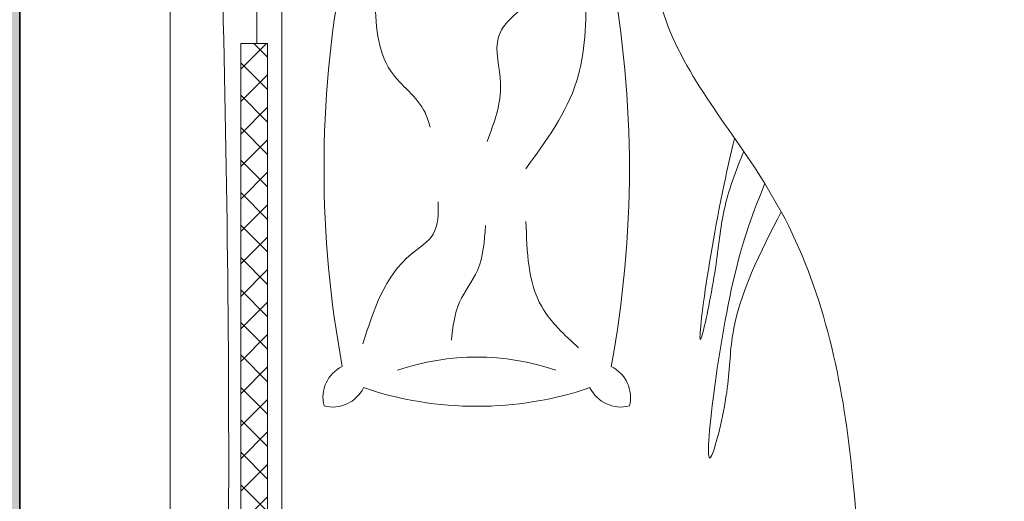
# Model space of a CAD drawing. Units: inches. Extents: x 2083 to 3317, y 1141 to 2115.
# Tile 96 of 256: x 2236 to 2290, y 1932 to 1958. Entities that reach past the tile are written whole.
import ezdxf

# ---------------------------------------------------------------- set-up
doc = ezdxf.new("R2010")
doc.units = ezdxf.units.IN
for name, color, linetype, lineweight in [('A-FURN', 8, 'Continuous', 18), ('A-WALL', 7, 'Continuous', 35), ('www.cadblocksfree.com', 7, 'Continuous', 9)]:
    doc.layers.add(name, color=color, linetype=linetype, lineweight=lineweight)
doc.layers.add('A-WALL-PATT', color=251, linetype='Continuous', lineweight=13, true_color=0x636466)

# ---------------------------------------------------------------- blocks, each defined once
blk = doc.blocks.new('bed')
at = {"layer": 'www.cadblocksfree.com', "ltscale": 0.2}
h = blk.add_hatch(dxfattribs=at)
h.set_pattern_fill('ANSI37,_O', color=256, scale=0.393701)
h.set_pattern_definition([(45, (2420.7222, -262.9689), (-0.8838835, 0.8838835), []), (135, (2420.7222, -262.9689), (-0.8838835, -0.8838835), [])])
h.paths.add_polyline_path([(3417.573, 1472.402), (3372.192, 1472.402), (3372.192, 1470.941), (3417.573, 1470.941)])
for p, q in [((3372.192, 1472.402), (3417.573, 1472.402)), ((3417.573, 1470.941), (3417.573, 1472.402)), ((3372.192, 1470.941), (3417.573, 1470.941)), ((3409.943, 1443.853), (3408.408, 1442.961))]:
    blk.add_line(p, q, dxfattribs=at)
for points in [[(3426.763, 1476.249), (3363.002, 1476.249)], [(3417.573, 1471.524), (3428.347, 1471.524), (3428.347, 1473.886)], [(3426.379, 1449.413), (3426.379, 1470.154), (3363.387, 1470.154), (3363.387, 1447.076)]]:
    blk.add_lwpolyline(points, dxfattribs=at)
for centre, radius, start, end in [((3394.883, 2431.358), 958.303, 268.093559, 271.906441), ((3399.641, 1467.396), 1.87, 165.5166, 244.2099), ((3398.298, 1466.054), 1.87, 25.7901, 104.4834), ((3410.752, 1409.187), 58.677, 79.42346, 100.57654), ((3417.027, 1459.547), 19.215, 161.2852, 198.7148), ((3387.154, 1459.547), 13.338, 341.1598, 18.8402), ((3399.641, 1451.698), 1.87, 115.7901, 194.4834), ((3398.298, 1453.041), 1.87, 255.5166, 334.2099), ((3410.752, 1509.907), 58.677, 259.42346, 280.57654)]:
    blk.add_arc(centre, radius, start, end, dxfattribs=at)
for points, knots in [([(3401.221, 1465.744), (3403.047, 1465.161), (3405.408, 1464.407), (3407.088, 1461.635), (3408.312, 1461.638), (3408.953, 1461.64)], [0, 0, 0, 0, 5.530688, 7.154877, 8.940839, 8.940839, 8.940839, 8.940839]), ([(3420.141, 1465.083), (3418.661, 1465.041), (3416.141, 1464.969), (3414.502, 1462.52), (3413.283, 1462.165), (3413.011, 1462.086)], [0, 0, 0, 0, 4.163459, 7.093919, 7.934624, 7.934624, 7.934624, 7.934624]), ([(3401.408, 1460.927), (3402.126, 1460.846), (3403.512, 1460.689), (3405.283, 1459.224), (3406.806, 1459.127), (3407.654, 1459.073)], [0, 0, 0, 0, 2.127543, 4.10272, 6.58647, 6.58647, 6.58647, 6.58647]), ([(3419.716, 1456.774), (3419.174, 1457.459), (3418.052, 1458.876), (3415.084, 1457.893), (3413.26, 1458.594), (3412.241, 1458.985)], [0, 0, 0, 0, 2.388143, 4.935423, 8.166198, 8.166198, 8.166198, 8.166198]), ([(3400.996, 1453.995), (3401.698, 1454.761), (3403.498, 1456.726), (3406.222, 1456.811), (3407.884, 1456.863)], [0, 0, 0, 0, 3.013696, 7.735839, 7.735839, 7.735839, 7.735839]), ([(3420.479, 1453.579), (3418.77, 1453.599), (3415.179, 1453.639), (3412.269, 1455.762), (3410.745, 1456.874)], [0, 0, 0, 0, 5.002087, 10.507046, 10.507046, 10.507046, 10.507046]), ([(3409.943, 1443.853), (3413.12, 1445.837), (3417.433, 1449.66), (3422.724, 1450.042), (3424.477, 1449.98)], [1.3582378, 1.3582378, 1.3582378, 1.3582378, 1.6381418, 1.7706953, 1.7706953, 1.7706953, 1.7706953]), ([(3412.402, 1445.499), (3411.605, 1445.698), (3406.242, 1446.932), (3398.173, 1447.93), (3405.397, 1446.464), (3408.571, 1446.191), (3410.626, 1445.456), (3411.681, 1445)], [0.1043639, 0.1043639, 0.1043639, 0.1043639, 0.1489731, 0.3882761, 0.4793617, 0.5593494, 0.6446217, 0.6446217, 0.6446217, 0.6446217]), ([(3409.943, 1443.853), (3408.469, 1444.451), (3404.443, 1446.042), (3391.397, 1447.599), (3398.64, 1445.767), (3402.973, 1445.759), (3406.219, 1444.095), (3408.408, 1442.961)], [0.0056315, 0.0056315, 0.0056315, 0.0056315, 0.1489731, 0.3882761, 0.4793617, 0.5593494, 0.7397317, 0.7397317, 0.7397317, 0.7397317]), ([(3362.928, 1430.813), (3365.944, 1432.958), (3375.455, 1438.993), (3392.12, 1438.03), (3404.249, 1440.73), (3408.408, 1442.961)], [0.102872, 0.102872, 0.102872, 0.102872, 0.37972, 0.957702, 1.313793, 1.313793, 1.313793, 1.313793])]:
    blk.add_open_spline(points, degree=3, knots=knots, dxfattribs=at)

msp = doc.modelspace()

# ---------------------------------------------------------------- hatches: boundary and pattern name
at = {"layer": 'A-WALL-PATT'}
h = msp.add_hatch(color=256, dxfattribs=at)
h.dxf.hatch_style = 1
h.paths.add_polyline_path([(3126.96, 2020.761), (2748.96, 2020.761), (2604.96, 2020.761), (2226.96, 2020.761), (2226.96, 1702.761), (2466.96, 1702.761), (2466.96, 1582.761), (2418.96, 1582.761), (2418.96, 1477.761), (2226.96, 1477.761), (2226.96, 1263.261), (2544.96, 1263.261), (2544.96, 1411.761), (2604.96, 1411.761), (2685.96, 1411.761), (2685.96, 1420.761), (2604.96, 1420.761), (2604.96, 1573.761), (2604.96, 1702.761), (2604.96, 2011.761), (2748.96, 2011.761), (2748.96, 1702.761), (2862.96, 1702.761), (2862.96, 1621.761), (2871.96, 1621.761), (2871.96, 1702.761), (2883.96, 1702.761), (2883.96, 1706.939, -0.026459), (2883.96, 1711.761), (2757.96, 1711.761), (2757.96, 1807.761), (2787.96, 1807.761), (2787.96, 1812.261), (2757.96, 1812.261), (2757.96, 2011.761), (2877.96, 2011.761), (2877.96, 1812.261), (2847.96, 1812.261), (2847.96, 1807.761), (2889.836, 1807.761), (2889.836, 1812.261), (2882.46, 1812.261), (2882.46, 2011.761), (3117.96, 2011.761), (3117.96, 1812.261), (2937.836, 1812.261), (2937.836, 1807.761), (2995.71, 1807.761), (2995.71, 1796.118), (3000.21, 1796.118), (3000.21, 1807.761), (3117.96, 1807.761), (3117.96, 1711.761), (3000.21, 1711.761), (3000.21, 1760.118), (2998.573, 1760.118, -0.020711), (2995.71, 1760.118), (2995.71, 1711.761), (2931.96, 1711.761), (2931.96, 1702.761), (3126.96, 1702.761)])
h.paths.add_polyline_path([(2471.46, 2011.761), (2471.46, 1810.011), (2462.717, 1810.011), (2462.717, 1805.511), (2505.96, 1805.511), (2505.96, 1810.011), (2475.96, 1810.011), (2475.96, 2011.761), (2595.96, 2011.761), (2595.96, 1810.011), (2565.96, 1810.011), (2565.96, 1805.511), (2595.96, 1805.511), (2595.96, 1711.761), (2235.96, 1711.761), (2235.96, 1805.511), (2353.71, 1805.511), (2353.71, 1796.054), (2358.21, 1796.054), (2358.21, 1805.511), (2414.717, 1805.511), (2414.717, 1810.011), (2235.96, 1810.011), (2235.96, 2011.761)], flags=16)
h.paths.add_polyline_path([(2270.205, 1994.61), (2270.205, 1970.61), (2246.205, 1970.61), (2246.205, 1994.61)], flags=0)
edge = h.paths.add_edge_path(flags=0)
edge.add_ellipse((2332.027, 1899.798), major_axis=(-3.043, 3.043), ratio=0.168252, start_angle=-161.3322, end_angle=-156.3071, ccw=False)
edge.add_ellipse((2333.082, 1898.744), major_axis=(-1.055, 1.055), ratio=0.453532, start_angle=-123.371, end_angle=-94.1591)
edge = h.paths.add_edge_path(flags=0)
edge.add_ellipse((2332.027, 1968.876), major_axis=(3.043, 3.043), ratio=0.168252, start_angle=18.6678, end_angle=23.6929)
edge.add_spline(control_points=[(2332.926, 1970.691), (2332.227, 1970.336), (2330.894, 1969.659), (2328.413, 1970.932), (2327.204, 1967.749), (2324.71, 1969.956), (2322.533, 1967.012), (2320.013, 1971.296), (2317.68, 1968.158), (2316.041, 1967.102), (2315.427, 1966.81)], knot_values=[0, 0, 0, 0, 2.267059, 4.324559, 6.685584, 8.878641, 11.121502, 14.300359, 17.755284, 19.732645, 19.732645, 19.732645, 19.732645], degree=3, periodic=0)
edge.add_ellipse((2332.027, 1968.876), major_axis=(3.043, 3.043), ratio=0.168252, start_angle=18.6678, end_angle=23.6929, ccw=False)
edge.add_ellipse((2333.082, 1969.931), major_axis=(1.055, 1.055), ratio=0.453532, start_angle=56.629, end_angle=85.8409, ccw=False)
edge = h.paths.add_edge_path(flags=0)
edge.add_spline(control_points=[(2296.428, 1967.988), (2293.628, 1965.336), (2287.704, 1959.727), (2299.744, 1949.996), (2294.533, 1935.669), (2290.573, 1920.604), (2293.394, 1909.974), (2296.185, 1904.967)], knot_values=[0.099185, 0.099185, 0.099185, 0.099185, 0.345301, 0.619822, 0.982653, 1.386093, 1.810555, 1.810555, 1.810555, 1.810555], degree=3, periodic=0)
edge.add_spline(control_points=[(2296.185, 1904.967), (2297.384, 1902.619), (2298.001, 1901.949), (2298.553, 1901.468)], knot_values=[0.006246, 0.006246, 0.006246, 0.006246, 0.055476, 0.055476, 0.055476, 0.055476], degree=3, periodic=0)
edge.add_spline(control_points=[(2298.553, 1901.468), (2297.259, 1900.923), (2295.225, 1900.232), (2293.06, 1900.614), (2292.101, 1900.788), (2292.09, 1900.791)], knot_values=[0.312835, 0.312835, 0.312835, 0.312835, 0.40178, 0.474987, 0.475903, 0.475903, 0.475903, 0.475903], degree=3, periodic=0)
edge.add_arc((2292.794, 1904.664), 3.937, 215.4209, 259.6982, ccw=False)
edge.add_spline(control_points=[(2289.585, 1902.382), (2289.477, 1902.535), (2289.368, 1902.688), (2289.261, 1902.841)], knot_values=[0.102872, 0.102872, 0.102872, 0.102872, 0.116896, 0.116896, 0.116896, 0.116896], degree=3, periodic=0)
edge.add_spline(control_points=[(2289.261, 1902.841), (2288.687, 1902.55), (2287.64, 1902.02), (2285.881, 1901.874), (2283.853, 1901.504), (2281.72, 1899.711), (2278.467, 1899.493), (2276.157, 1901.883), (2272.259, 1899.804), (2267.778, 1901.843), (2262.244, 1900.184), (2257.415, 1901.782), (2254.318, 1900.726), (2253.178, 1900.337)], knot_values=[0, 0, 0, 0, 1.907977, 3.477176, 5.261074, 7.972851, 11.680248, 13.717921, 16.939592, 22.789562, 27.502503, 33.595215, 37.145618, 37.145618, 37.145618, 37.145618], degree=3, periodic=0)
edge.add_line((2253.178, 1900.337), (2250.244, 1902.841))
edge.add_line((2250.244, 1902.841), (2250.244, 1965.833))
edge.add_line((2250.244, 1965.833), (2253.178, 1968.337))
edge.add_spline(control_points=[(2253.178, 1968.337), (2254.318, 1967.948), (2257.415, 1966.892), (2262.244, 1968.49), (2267.778, 1966.831), (2271.527, 1968.537), (2273.876, 1967.828), (2274.207, 1967.728)], knot_values=[0, 0, 0, 0, 0.09018, 0.244935, 0.364644, 0.513233, 0.537855, 0.537855, 0.537855, 0.537855], degree=3, periodic=0)
edge.add_arc((2274.353, 1963.793), 3.937, 72.0511, 92.1279, ccw=False)
edge.add_arc((2281.297, 1985.23), 18.596, 252.0511, 288.5657)
edge.add_arc((2292.317, 1956.029), 12.646, 71.0268, 113.7782, ccw=False)
edge = h.paths.add_edge_path(flags=0)
edge.add_spline(control_points=[(2274.899, 1951.856), (2275.066, 1951.617), (2275.233, 1951.377), (2275.398, 1951.136)], knot_values=[1.409916, 1.409916, 1.409916, 1.409916, 1.43159, 1.43159, 1.43159, 1.43159], degree=3, periodic=0)
edge.add_spline(control_points=[(2275.398, 1951.136), (2275.792, 1950.562), (2276.179, 1949.984), (2276.546, 1949.397)], knot_values=[1.358238, 1.358238, 1.358238, 1.358238, 1.409916, 1.409916, 1.409916, 1.409916], degree=3, periodic=0)
edge.add_line((2276.546, 1949.397), (2277.437, 1947.862))
edge.add_spline(control_points=[(2277.437, 1947.862), (2276.304, 1945.673), (2274.64, 1942.427), (2274.632, 1938.094), (2272.799, 1930.852), (2274.356, 1943.897), (2275.948, 1947.923), (2276.546, 1949.397)], knot_values=[0.005632, 0.005632, 0.005632, 0.005632, 0.186014, 0.266002, 0.357087, 0.59639, 0.739732, 0.739732, 0.739732, 0.739732], degree=3, periodic=0)
edge.add_spline(control_points=[(2276.546, 1949.397), (2276.179, 1949.984), (2275.792, 1950.562), (2275.398, 1951.136)], knot_values=[1.358238, 1.358238, 1.358238, 1.358238, 1.409916, 1.409916, 1.409916, 1.409916], degree=3, periodic=0)
edge.add_spline(control_points=[(2275.398, 1951.136), (2274.943, 1950.08), (2274.208, 1948.025), (2273.935, 1944.851), (2272.469, 1937.627), (2273.466, 1945.696), (2274.701, 1951.059), (2274.899, 1951.856)], knot_values=[0.104364, 0.104364, 0.104364, 0.104364, 0.189636, 0.269624, 0.36071, 0.600013, 0.644622, 0.644622, 0.644622, 0.644622], degree=3, periodic=0)
h.paths.add_polyline_path([(2269.168, 1963.128, -0.357527), (2268.171, 1960.976, -0.092561), (2268.171, 1939.436, -0.357527), (2269.168, 1937.285, -0.357527), (2267.016, 1938.282, -0.164785), (2254.686, 1938.282, -0.357527), (2252.534, 1937.285, -0.357527), (2253.531, 1939.436, -0.092561), (2253.531, 1960.976, -0.357527), (2252.534, 1963.128, -0.357527), (2254.686, 1962.131, -0.164785), (2267.016, 1962.131, -0.357527)], flags=0)
h.paths.add_polyline_path([(2248.874, 1967.802), (2248.874, 1957.028), (2249.458, 1957.028), (2249.458, 1911.647), (2248.874, 1911.647), (2248.874, 1900.873), (2246.512, 1900.873, 0.197327), (2244.15, 1902.457), (2244.15, 1966.218, 0.197327), (2246.512, 1967.802)], flags=0)
h.paths.add_polyline_path([(2269.168, 1931.389, -0.357527), (2268.171, 1929.238, -0.092561), (2268.171, 1907.698, -0.357527), (2269.168, 1905.547, -0.357527), (2267.016, 1906.544, -0.164785), (2254.686, 1906.544, -0.357527), (2252.534, 1905.547, -0.357527), (2253.531, 1907.698, -0.092561), (2253.531, 1929.238, -0.357527), (2252.534, 1931.389, -0.357527), (2254.686, 1930.392, -0.164785), (2267.016, 1930.392, -0.357527)], flags=0)
edge = h.paths.add_edge_path(flags=0)
edge.add_spline(control_points=[(2276.197, 1906.724), (2276.168, 1909.029), (2276.114, 1913.372), (2270.598, 1924.925), (2273.905, 1919.013), (2275.922, 1916.262), (2275.475, 1912.402), (2277.258, 1910.381), (2276.696, 1908.225), (2276.646, 1906.813), (2276.618, 1906.008)], knot_values=[0, 0, 0, 0, 8.61026, 16.221274, 18.843057, 23.804898, 27.440828, 29.356102, 31.203478, 33.650687, 33.650687, 33.650687, 33.650687], degree=3, periodic=0)
edge.add_spline(control_points=[(2276.618, 1906.008), (2276.623, 1905.624), (2276.498, 1904.629), (2275.442, 1903.855), (2274.937, 1903.08), (2274.859, 1902.841)], knot_values=[0.156488, 0.156488, 0.156488, 0.156488, 0.184398, 0.231376, 0.250598, 0.250598, 0.250598, 0.250598], degree=3, periodic=0)
edge.add_line((2274.859, 1902.841), (2276.506, 1902.841))
edge.add_spline(control_points=[(2276.506, 1902.841), (2276.788, 1903.085), (2277.665, 1904.125), (2278.25, 1904.341), (2277.654, 1908.527), (2278.156, 1906.228), (2278.1, 1905.286), (2278.847, 1904.069), (2277.857, 1903.415), (2277.874, 1902.991), (2277.904, 1902.841)], knot_values=[0.059574, 0.059574, 0.059574, 0.059574, 0.080753, 0.103741, 0.16972, 0.176036, 0.207137, 0.240474, 0.262341, 0.27366, 0.27366, 0.27366, 0.27366], degree=3, periodic=0)
edge.add_line((2277.904, 1902.841), (2280.03, 1902.841))
edge.add_spline(control_points=[(2280.03, 1902.841), (2279.888, 1903.088), (2279.499, 1903.982), (2280.152, 1905.939), (2278.104, 1909.658), (2279.762, 1907.185), (2280.328, 1904.875), (2280.485, 1903.49), (2281.463, 1903.249), (2281.758, 1902.936), (2281.834, 1902.841)], knot_values=[0.013856, 0.013856, 0.013856, 0.013856, 0.034874, 0.088867, 0.107879, 0.126738, 0.158714, 0.193757, 0.217487, 0.226722, 0.226722, 0.226722, 0.226722], degree=3, periodic=0)
edge.add_spline(control_points=[(2281.834, 1902.841), (2281.788, 1902.827), (2281.647, 1902.783), (2281.396, 1902.859), (2281.088, 1902.985), (2280.721, 1903.061), (2280.333, 1903.026), (2280.125, 1902.899), (2280.03, 1902.841)], knot_values=[0, 0, 0, 0, 0.14413, 0.435517, 0.749276, 1.153046, 1.548371, 1.878348, 1.878348, 1.878348, 1.878348], degree=3, periodic=0)
edge.add_line((2280.03, 1902.841), (2277.904, 1902.841))
edge.add_spline(control_points=[(2277.904, 1902.841), (2277.893, 1902.796), (2277.865, 1902.68), (2277.607, 1902.687), (2277.274, 1902.801), (2276.838, 1902.62), (2276.584, 1902.789), (2276.506, 1902.841)], knot_values=[0, 0, 0, 0, 0.127189, 0.326199, 0.628009, 1.24357, 1.515331, 1.515331, 1.515331, 1.515331], degree=3, periodic=0)
edge.add_line((2276.506, 1902.841), (2274.859, 1902.841))
edge.add_spline(control_points=[(2274.859, 1902.841), (2274.814, 1902.899), (2274.725, 1903.013), (2274.493, 1903.119), (2274.244, 1902.961), (2273.937, 1903.185), (2273.614, 1902.983), (2273.408, 1902.883), (2273.322, 1902.841)], knot_values=[0, 0, 0, 0, 0.21843, 0.436957, 0.687977, 0.990379, 1.398396, 1.69185, 1.69185, 1.69185, 1.69185], degree=3, periodic=0)
edge.add_spline(control_points=[(2273.322, 1902.841), (2273.617, 1903.446), (2274.274, 1904.538), (2276.027, 1904.574), (2276.207, 1906.584), (2276.197, 1906.724)], knot_values=[0.012227, 0.012227, 0.012227, 0.012227, 0.059472, 0.106218, 0.134458, 0.134458, 0.134458, 0.134458], degree=3, periodic=0)
h.paths.add_polyline_path([(2270.776, 1897.79), (2270.776, 1873.79), (2246.776, 1873.79), (2246.776, 1897.79)], flags=0)
h.paths.add_polyline_path([(2353.71, 1760.005), (2353.71, 1760.054), (2358.21, 1760.054, -0.033729)], flags=0)
h.paths.add_polyline_path([(2321.819, 1737.529), (2341.995, 1737.529, -0.414214), (2343.203, 1736.321), (2343.203, 1721.021, -0.414214), (2341.995, 1719.813), (2321.819, 1719.813, -0.414214), (2320.611, 1721.021), (2320.611, 1736.321, -0.414214)], flags=0)
h.paths.add_polyline_path([(2324.235, 1736.321), (2339.579, 1736.321, -0.414214), (2341.995, 1733.905), (2341.995, 1725.45, -0.414214), (2339.579, 1723.034), (2333.681, 1723.034), (2333.845, 1722.045, -0.870646), (2335.425, 1721.826, -0.767327), (2333.923, 1721.423), (2331.291, 1721.423, -0.767327), (2329.788, 1721.826, -0.870646), (2331.368, 1722.045), (2331.533, 1723.034), (2324.235, 1723.034, -0.414214), (2321.819, 1725.45), (2321.819, 1733.905, -0.414214)], flags=0)
h.paths.add_polyline_path([(2570.484, 1928.615), (2589.684, 1928.615), (2590.169, 1928.615), (2590.169, 1904.993), (2570.484, 1904.993)], flags=0)
h.paths.add_polyline_path([(2574.447, 1927.264, -1), (2572.829, 1927.264, -1)], flags=0)
h.paths.add_polyline_path([(2573.09, 1926.941), (2573.925, 1927.776), (2574.148, 1927.553), (2573.313, 1926.718)], flags=0)
h.paths.add_polyline_path([(2578.779, 1919.73, -1), (2571.592, 1919.73, -1)], flags=0)
h.paths.add_polyline_path([(2578.385, 1919.73, -1), (2571.985, 1919.73, -1)], flags=0)
h.paths.add_polyline_path([(2331.596, 1729.476, -1), (2333.618, 1729.476, -1)], flags=0)
h.paths.add_polyline_path([(2578.034, 1927.264, -1), (2576.416, 1927.264, -1)], flags=0)
h.paths.add_polyline_path([(2576.689, 1927.531), (2576.912, 1927.754), (2577.747, 1926.919), (2577.524, 1926.696)], flags=0)
h.paths.add_polyline_path([(2578.139, 1909.86, -1), (2572.232, 1909.86, -1)], flags=0)
h.paths.add_polyline_path([(2577.745, 1909.86, -1), (2572.625, 1909.86, -1)], flags=0)
h.paths.add_polyline_path([(2583.798, 1927.264, -1), (2582.179, 1927.264, -1)], flags=0)
h.paths.add_polyline_path([(2582.719, 1927.754), (2583.554, 1926.919), (2583.331, 1926.696), (2582.496, 1927.531)], flags=0)
h.paths.add_polyline_path([(2582.496, 1927.531), (2582.719, 1927.754), (2583.554, 1926.919), (2583.331, 1926.696)], flags=0)
h.paths.add_polyline_path([(2587.739, 1920.53, -1), (2581.832, 1920.53, -1)], flags=0)
h.paths.add_polyline_path([(2587.345, 1920.53, -1), (2582.225, 1920.53, -1)], flags=0)
h.paths.add_polyline_path([(2587.385, 1927.264, -1), (2585.766, 1927.264, -1)], flags=0)
h.paths.add_polyline_path([(2586.082, 1926.98), (2586.917, 1927.815), (2587.14, 1927.593), (2586.305, 1926.758)], flags=0)
h.paths.add_polyline_path([(2588.379, 1910.66, -1), (2581.192, 1910.66, -1)], flags=0)
h.paths.add_polyline_path([(2587.985, 1910.66, -1), (2581.585, 1910.66, -1)], flags=0)
h.paths.add_polyline_path([(2417.168, 1729.478), (2437.344, 1729.478, -0.414214), (2438.552, 1728.27), (2438.552, 1712.969, -0.414214), (2437.344, 1711.761), (2417.168, 1711.761, -0.414214), (2415.96, 1712.969), (2415.96, 1728.27, -0.414214)], flags=0)
h.paths.add_polyline_path([(2419.584, 1728.27), (2434.928, 1728.27, -0.414214), (2437.344, 1725.854), (2437.344, 1717.398, -0.414214), (2434.928, 1714.983), (2429.029, 1714.983), (2429.194, 1713.994, -0.870646), (2430.774, 1713.775, -0.767327), (2429.271, 1713.372), (2426.64, 1713.372, -0.767327), (2425.137, 1713.775, -0.870646), (2426.717, 1713.994), (2426.882, 1714.983), (2419.584, 1714.983, -0.414214), (2417.168, 1717.398), (2417.168, 1725.854, -0.414214)], flags=0)
h.paths.add_polyline_path([(2419.584, 1728.27), (2434.928, 1728.27, -0.414214), (2437.344, 1725.854), (2437.344, 1717.398, -0.414214), (2434.928, 1714.983), (2429.029, 1714.983), (2428.358, 1719.009), (2427.553, 1719.009), (2426.882, 1714.983), (2419.584, 1714.983, -0.414214), (2417.168, 1717.398), (2417.168, 1725.854, -0.414214)], flags=0)
h.paths.add_polyline_path([(2426.944, 1721.425, -1), (2428.967, 1721.425, -1)], flags=0)
h.paths.add_polyline_path([(2475.96, 1702.761), (2595.96, 1702.761), (2595.96, 1582.761), (2475.96, 1582.761)], flags=16)
h.paths.add_polyline_path([(2427.96, 1573.761), (2595.96, 1573.761), (2595.96, 1468.761), (2595.96, 1420.761), (2384.46, 1420.761), (2384.46, 1468.761), (2427.96, 1468.761)], flags=16)
h.paths.add_polyline_path([(2379.96, 1468.761), (2379.96, 1420.761), (2235.96, 1420.761), (2235.96, 1468.761)], flags=16)
h.paths.add_polyline_path([(2317.816, 1466.696), (2337.992, 1466.696, -0.414214), (2339.2, 1465.488), (2339.2, 1450.187, -0.414214), (2337.992, 1448.979), (2317.816, 1448.979, -0.414214), (2316.608, 1450.187), (2316.608, 1465.488, -0.414214)], flags=0)
h.paths.add_polyline_path([(2320.232, 1465.488), (2335.576, 1465.488, -0.414214), (2337.992, 1463.072), (2337.992, 1454.616, -0.414214), (2335.576, 1452.2), (2329.677, 1452.2), (2329.842, 1451.212, -0.870646), (2331.422, 1450.992, -0.767327), (2329.92, 1450.59), (2327.288, 1450.59, -0.767327), (2325.785, 1450.992, -0.870646), (2327.365, 1451.212), (2327.53, 1452.2), (2320.232, 1452.2, -0.414214), (2317.816, 1454.616), (2317.816, 1463.072, -0.414214)], flags=0)
h.paths.add_polyline_path([(2320.232, 1465.488), (2335.576, 1465.488, -0.414214), (2337.992, 1463.072), (2337.992, 1454.616, -0.414214), (2335.576, 1452.2), (2329.677, 1452.2), (2329.006, 1456.227), (2328.201, 1456.227), (2327.53, 1452.2), (2320.232, 1452.2, -0.414214), (2317.816, 1454.616), (2317.816, 1463.072, -0.414214)], flags=0)
h.paths.add_polyline_path([(2327.593, 1458.643, -1), (2329.615, 1458.643, -1)], flags=0)
h.paths.add_polyline_path([(2244.412, 1433.34), (2241.921, 1433.34, -0.414214), (2240.018, 1435.244), (2240.018, 1440.953, -0.414211), (2241.921, 1442.856), (2244.412, 1442.856, -1.976472)], flags=0)
h.paths.add_polyline_path([(2245.357, 1434.398, -0.414214), (2245.357, 1441.799, -2.144098)], flags=0)
h.paths.add_polyline_path([(2535.96, 1416.261), (2535.96, 1272.261), (2235.96, 1272.261), (2235.96, 1416.261)], flags=16)
h.paths.add_polyline_path([(2260.12, 1384.293), (2260.12, 1362.039), (2237.865, 1362.039), (2237.865, 1384.293)], flags=0)
edge = h.paths.add_edge_path(flags=0)
edge.add_line((2318.252, 1362.093), (2318.146, 1362.001))
edge.add_ellipse((2317.445, 1360.431), major_axis=(2.822, 2.822), ratio=0.168252, start_angle=18.6678, end_angle=20.9481, ccw=False)
edge.add_ellipse((2318.423, 1361.409), major_axis=(0.978, 0.978), ratio=0.453532, start_angle=56.629, end_angle=70.2262, ccw=False)
edge = h.paths.add_edge_path(flags=0)
edge.add_line((2319.107, 1295.571), (2319.015, 1295.677))
edge.add_ellipse((2317.445, 1296.378), major_axis=(-2.822, 2.822), ratio=0.168252, start_angle=-161.3322, end_angle=-159.0519, ccw=False)
edge.add_ellipse((2318.423, 1295.4), major_axis=(-0.978, 0.978), ratio=0.453532, start_angle=-123.371, end_angle=-109.7738)
edge = h.paths.add_edge_path(flags=0)
edge.add_spline(control_points=[(2284.21, 1301.17), (2284.581, 1300.445), (2284.891, 1299.892), (2285.16, 1299.461)], knot_values=[0.039066, 0.039066, 0.039066, 0.039066, 0.055476, 0.055476, 0.055476, 0.055476], degree=3, periodic=0)
edge.add_line((2285.16, 1299.461), (2284.21, 1301.17))
edge = h.paths.add_edge_path(flags=0)
edge.add_line((2280.412, 1297.298), (2283.37, 1297.036))
edge.add_line((2283.37, 1297.036), (2286.406, 1297.926))
edge.add_spline(control_points=[(2286.406, 1297.926), (2285.305, 1297.463), (2284.345, 1297.129), (2283.37, 1297.036)], knot_values=[0.394369, 0.394369, 0.394369, 0.394369, 0.475903, 0.475903, 0.475903, 0.475903], degree=3, periodic=0)
edge.add_spline(control_points=[(2283.37, 1297.036), (2283.281, 1297.028), (2282.316, 1296.957), (2281.313, 1297.134), (2280.423, 1297.296), (2280.412, 1297.298)], knot_values=[0.312835, 0.312835, 0.312835, 0.312835, 0.320246, 0.393453, 0.394369, 0.394369, 0.394369, 0.394369], degree=3, periodic=0)
edge = h.paths.add_edge_path(flags=0)
edge.add_line((2284.436, 1359.607), (2280.446, 1355.328))
edge.add_line((2280.446, 1355.328), (2279.58, 1351.018))
edge.add_line((2279.58, 1351.018), (2282.413, 1346.58))
edge.add_spline(control_points=[(2282.413, 1346.58), (2283.153, 1345.589), (2284.253, 1344.029), (2284.801, 1342.387), (2284.935, 1341.806)], knot_values=[1.240098, 1.240098, 1.240098, 1.240098, 1.332892, 1.382712, 1.382712, 1.382712, 1.382712], degree=3, periodic=0)
edge.add_spline(control_points=[(2284.935, 1341.806), (2285.319, 1340.141), (2285.233, 1338.409), (2284.91, 1336.654)], knot_values=[1.097484, 1.097484, 1.097484, 1.097484, 1.240098, 1.240098, 1.240098, 1.240098], degree=3, periodic=0)
edge.add_spline(control_points=[(2284.91, 1336.654), (2284.587, 1334.899), (2284.027, 1333.12), (2283.463, 1331.361)], knot_values=[0.95487, 0.95487, 0.95487, 0.95487, 1.097484, 1.097484, 1.097484, 1.097484], degree=3, periodic=0)
edge.add_line((2283.463, 1331.361), (2281.89, 1326.153))
edge.add_line((2281.89, 1326.153), (2280.756, 1321.056))
edge.add_line((2280.756, 1321.056), (2280.299, 1316.002))
edge.add_line((2280.299, 1316.002), (2280.716, 1310.95))
edge.add_line((2280.716, 1310.95), (2282.028, 1305.972))
edge.add_line((2282.028, 1305.972), (2284.21, 1301.17))
edge.add_spline(control_points=[(2284.21, 1301.17), (2283.341, 1302.73), (2282.612, 1304.336), (2282.028, 1305.972)], knot_values=[0.099185, 0.099185, 0.099185, 0.099185, 0.241799, 0.241799, 0.241799, 0.241799], degree=3, periodic=0)
edge.add_spline(control_points=[(2282.028, 1305.972), (2281.444, 1307.608), (2281.005, 1309.273), (2280.716, 1310.95)], knot_values=[0.241799, 0.241799, 0.241799, 0.241799, 0.384413, 0.384413, 0.384413, 0.384413], degree=3, periodic=0)
edge.add_spline(control_points=[(2280.716, 1310.95), (2280.433, 1312.588), (2280.289, 1314.277), (2280.299, 1315.962), (2280.299, 1316.002)], knot_values=[0.384413, 0.384413, 0.384413, 0.384413, 0.523647, 0.527028, 0.527028, 0.527028, 0.527028], degree=3, periodic=0)
edge.add_spline(control_points=[(2280.299, 1316.002), (2280.312, 1317.687), (2280.478, 1319.368), (2280.756, 1321.056)], knot_values=[0.527028, 0.527028, 0.527028, 0.527028, 0.669642, 0.669642, 0.669642, 0.669642], degree=3, periodic=0)
edge.add_spline(control_points=[(2280.756, 1321.056), (2281.035, 1322.744), (2281.426, 1324.44), (2281.89, 1326.153)], knot_values=[0.669642, 0.669642, 0.669642, 0.669642, 0.812256, 0.812256, 0.812256, 0.812256], degree=3, periodic=0)
edge.add_spline(control_points=[(2281.89, 1326.153), (2282.264, 1327.533), (2282.788, 1329.262), (2283.353, 1331.018), (2283.463, 1331.361)], knot_values=[0.812256, 0.812256, 0.812256, 0.812256, 0.927087, 0.95487, 0.95487, 0.95487, 0.95487], degree=3, periodic=0)
edge.add_line((2283.463, 1331.361), (2284.91, 1336.654))
edge.add_line((2284.91, 1336.654), (2284.935, 1341.806))
edge.add_line((2284.935, 1341.806), (2282.413, 1346.58))
edge.add_spline(control_points=[(2282.413, 1346.58), (2281.275, 1348.104), (2280.078, 1349.57), (2279.58, 1351.018)], knot_values=[1.382712, 1.382712, 1.382712, 1.382712, 1.525326, 1.525326, 1.525326, 1.525326], degree=3, periodic=0)
edge.add_spline(control_points=[(2279.58, 1351.018), (2279.443, 1351.415), (2279.136, 1352.857), (2279.735, 1354.29), (2280.446, 1355.328)], knot_values=[1.525326, 1.525326, 1.525326, 1.525326, 1.564439, 1.667941, 1.667941, 1.667941, 1.667941], degree=3, periodic=0)
edge.add_spline(control_points=[(2280.446, 1355.328), (2281.426, 1356.758), (2282.931, 1358.183), (2284.436, 1359.607)], knot_values=[1.667941, 1.667941, 1.667941, 1.667941, 1.810555, 1.810555, 1.810555, 1.810555], degree=3, periodic=0)
edge.add_arc((2280.623, 1348.518), 11.726, 71.0268, 113.7782)
edge.add_arc((2270.405, 1375.595), 17.244, 252.0511, 288.5657, ccw=False)
edge.add_arc((2263.966, 1355.718), 3.651, 72.0511, 92.1279)
edge.add_arc((2263.966, 1355.718), 3.651, 92.1279, 177.9851)
edge.add_spline(control_points=[(2260.318, 1355.846), (2260.26, 1354.221), (2260.551, 1350.187), (2262.999, 1346.766), (2264.473, 1344.649)], knot_values=[1.43159, 1.43159, 1.43159, 1.43159, 1.564144, 1.770695, 1.770695, 1.770695, 1.770695], degree=3, periodic=0)
edge.add_line((2264.473, 1344.649), (2264.936, 1343.983))
edge.add_spline(control_points=[(2263.801, 1340.248), (2263.843, 1340.514), (2264.067, 1341.756), (2264.513, 1343.002), (2264.935, 1343.981)], knot_values=[0.53657, 0.53657, 0.53657, 0.53657, 0.559349, 0.644622, 0.644622, 0.644622, 0.644622], degree=3, periodic=0)
edge.add_spline(control_points=[(2264.935, 1343.981), (2265.118, 1343.715), (2265.299, 1343.448), (2265.477, 1343.179)], knot_values=[1.384077, 1.384077, 1.384077, 1.384077, 1.409916, 1.409916, 1.409916, 1.409916], degree=3, periodic=0)
edge.add_spline(control_points=[(2265.477, 1343.179), (2265.655, 1342.911), (2265.829, 1342.641), (2265.999, 1342.369)], knot_values=[1.358238, 1.358238, 1.358238, 1.358238, 1.384077, 1.384077, 1.384077, 1.384077], degree=3, periodic=0)
edge.add_line((2265.999, 1342.369), (2266.826, 1340.946))
edge.add_spline(control_points=[(2266.826, 1340.946), (2268.894, 1337.09), (2271.398, 1325.843), (2270.516, 1310.569), (2275.919, 1301.861), (2277.79, 1299.199)], knot_values=[0.116896, 0.116896, 0.116896, 0.116896, 0.472987, 1.050969, 1.313793, 1.313793, 1.313793, 1.313793], degree=3, periodic=0)
edge.add_spline(control_points=[(2277.79, 1299.199), (2277.839, 1299.128), (2277.889, 1299.057), (2277.94, 1298.987)], knot_values=[0.109884, 0.109884, 0.109884, 0.109884, 0.116896, 0.116896, 0.116896, 0.116896], degree=3, periodic=0)
edge.add_line((2277.94, 1298.987), (2277.789, 1299.199))
edge.add_spline(control_points=[(2277.789, 1299.199), (2277.257, 1298.929), (2276.286, 1298.438), (2275.039, 1298.334), (2274.383, 1298.239), (2274.215, 1298.209)], knot_values=[33.12187, 33.12187, 33.12187, 33.12187, 35.029056, 36.598255, 37.144827, 37.144827, 37.144827, 37.144827], degree=3, periodic=0)
edge.add_line((2274.215, 1298.209), (2273.073, 1297.893))
edge.add_spline(control_points=[(2273.073, 1297.893), (2272.323, 1297.58), (2271.039, 1296.511), (2269.248, 1296.226), (2268.423, 1296.375)], knot_values=[26.532584, 26.532584, 26.532584, 26.532584, 29.198919, 31.839101, 31.839101, 31.839101, 31.839101], degree=3, periodic=0)
edge.add_line((2268.423, 1296.375), (2263.879, 1297.458))
edge.add_spline(control_points=[(2263.879, 1297.458), (2263.556, 1297.359), (2261.86, 1296.839), (2260.239, 1297.282), (2258.933, 1297.516)], knot_values=[15.919551, 15.919551, 15.919551, 15.919551, 16.939592, 21.226067, 21.226067, 21.226067, 21.226067], degree=3, periodic=0)
edge.add_line((2258.933, 1297.516), (2254.055, 1297.329))
edge.add_spline(control_points=[(2254.055, 1297.329), (2253.756, 1297.296), (2252.114, 1297.165), (2250.462, 1297.544), (2249.13, 1297.668)], knot_values=[5.306517, 5.306517, 5.306517, 5.306517, 6.276435, 10.613034, 10.613034, 10.613034, 10.613034], degree=3, periodic=0)
edge.add_line((2249.13, 1297.668), (2244.332, 1296.878))
edge.add_line((2244.332, 1296.878), (2241.611, 1299.199))
edge.add_line((2241.611, 1299.199), (2241.611, 1357.609))
edge.add_line((2241.611, 1357.609), (2244.332, 1359.931))
edge.add_line((2244.332, 1359.931), (2252.729, 1359.543))
edge.add_spline(control_points=[(2252.729, 1359.543), (2252.871, 1359.546), (2253.306, 1359.548), (2253.74, 1359.514), (2254.032, 1359.482)], knot_values=[0.233291, 0.233291, 0.233291, 0.233291, 0.244935, 0.268927, 0.268927, 0.268927, 0.268927], degree=3, periodic=0)
edge.add_line((2254.032, 1359.482), (2259.587, 1359.416))
edge.add_spline(control_points=[(2259.587, 1359.416), (2260.677, 1359.629), (2262.073, 1359.897), (2263.524, 1359.459), (2263.83, 1359.366)], knot_values=[0.422516, 0.422516, 0.422516, 0.422516, 0.513233, 0.537855, 0.537855, 0.537855, 0.537855], degree=3, periodic=0)
edge.add_arc((2263.966, 1355.718), 3.651, 72.0511, 92.1279, ccw=False)
edge.add_arc((2270.405, 1375.595), 17.244, 252.0511, 288.5657)
edge.add_arc((2280.623, 1348.518), 11.726, 71.0268, 113.7782, ccw=False)
h.paths.add_polyline_path([(2240.341, 1359.435), (2240.341, 1349.444), (2240.882, 1349.444), (2240.882, 1307.365), (2240.341, 1307.365), (2240.341, 1297.374), (2238.15, 1297.374, 0.197327), (2235.96, 1298.843), (2235.96, 1357.966, 0.197327), (2238.15, 1359.435)], flags=0)
h.paths.add_polyline_path([(2259.158, 1355.101, -0.357527), (2258.233, 1353.106, -0.092561), (2258.233, 1333.133, -0.357527), (2259.158, 1331.138, -0.357527), (2257.163, 1332.062, -0.164785), (2245.729, 1332.062, -0.357527), (2243.735, 1331.138, -0.357527), (2244.659, 1333.133, -0.092561), (2244.659, 1353.106, -0.357527), (2243.735, 1355.101, -0.357527), (2245.729, 1354.176, -0.164785), (2257.163, 1354.176, -0.357527)], flags=0)
edge = h.paths.add_edge_path(flags=0)
edge.add_line((2265.999, 1342.369), (2266.826, 1340.946))
edge.add_line((2266.826, 1340.946), (2265.308, 1337.814))
edge.add_line((2265.308, 1337.814), (2264.358, 1334.653))
edge.add_line((2264.358, 1334.653), (2264.262, 1333.8))
edge.add_spline(control_points=[(2264.262, 1333.8), (2264.208, 1333.187), (2264.162, 1332.366), (2264.007, 1331.414), (2263.969, 1331.202)], knot_values=[0.464444, 0.464444, 0.464444, 0.464444, 0.516691, 0.531608, 0.531608, 0.531608, 0.531608], degree=3, periodic=0)
edge.add_spline(control_points=[(2263.969, 1331.202), (2263.775, 1330.119), (2263.424, 1328.791), (2263.257, 1328.531), (2263.234, 1328.515)], knot_values=[0.372682, 0.372682, 0.372682, 0.372682, 0.44885, 0.464444, 0.464444, 0.464444, 0.464444], degree=3, periodic=0)
edge.add_spline(control_points=[(2263.234, 1328.515), (2263.096, 1328.42), (2263.131, 1329.301), (2263.275, 1330.616)], knot_values=[0.280919, 0.280919, 0.280919, 0.280919, 0.372682, 0.372682, 0.372682, 0.372682], degree=3, periodic=0)
edge.add_spline(control_points=[(2263.275, 1330.616), (2263.419, 1331.93), (2263.672, 1333.677), (2263.97, 1335.315)], knot_values=[0.189157, 0.189157, 0.189157, 0.189157, 0.280919, 0.280919, 0.280919, 0.280919], degree=3, periodic=0)
edge.add_spline(control_points=[(2263.97, 1335.315), (2264.1, 1336.032), (2264.419, 1337.622), (2264.755, 1338.864), (2264.947, 1339.491)], knot_values=[0.097394, 0.097394, 0.097394, 0.097394, 0.137578, 0.189157, 0.189157, 0.189157, 0.189157], degree=3, periodic=0)
edge.add_spline(control_points=[(2264.947, 1339.491), (2265.29, 1340.606), (2265.644, 1341.494), (2265.999, 1342.369)], knot_values=[0.005632, 0.005632, 0.005632, 0.005632, 0.097394, 0.097394, 0.097394, 0.097394], degree=3, periodic=0)
h.paths.add_polyline_path([(2259.158, 1325.671, -0.357527), (2258.233, 1323.676, -0.092561), (2258.233, 1303.703, -0.357527), (2259.158, 1301.708, -0.357527), (2257.163, 1302.633, -0.164785), (2245.729, 1302.633, -0.357527), (2243.735, 1301.708, -0.357527), (2244.659, 1303.703, -0.092561), (2244.659, 1323.676, -0.357527), (2243.735, 1325.671, -0.357527), (2245.729, 1324.747, -0.164785), (2257.163, 1324.747, -0.357527)], flags=0)
edge = h.paths.add_edge_path(flags=0)
edge.add_spline(control_points=[(2261.709, 1317.311), (2261.679, 1317.418), (2261.762, 1317.389), (2262.491, 1316.09), (2262.962, 1315.301)], knot_values=[14.955861, 14.955861, 14.955861, 14.955861, 16.221274, 18.694826, 18.694826, 18.694826, 18.694826], degree=3, periodic=0)
edge.add_spline(control_points=[(2262.962, 1315.301), (2262.99, 1315.254), (2263.702, 1314.067), (2264.349, 1313.127), (2264.73, 1312.164)], knot_values=[18.694826, 18.694826, 18.694826, 18.694826, 18.843057, 22.433791, 22.433791, 22.433791, 22.433791], degree=3, periodic=0)
edge.add_spline(control_points=[(2264.73, 1312.164), (2264.876, 1311.796), (2265.177, 1310.77), (2265.143, 1309.559), (2265.248, 1308.824)], knot_values=[22.433791, 22.433791, 22.433791, 22.433791, 23.804898, 26.172756, 26.172756, 26.172756, 26.172756], degree=3, periodic=0)
edge.add_line((2265.248, 1308.824), (2265.851, 1307.172))
edge.add_spline(control_points=[(2265.851, 1307.172), (2266.065, 1306.822), (2266.384, 1306.332), (2266.424, 1305.781), (2266.42, 1305.611)], knot_values=[28.062562, 28.062562, 28.062562, 28.062562, 29.356102, 29.911721, 29.911721, 29.911721, 29.911721], degree=3, periodic=0)
edge.add_spline(control_points=[(2266.42, 1305.611), (2266.416, 1305.433), (2266.394, 1305.25), (2266.365, 1305.066)], knot_values=[29.911721, 29.911721, 29.911721, 29.911721, 30.497837, 30.497837, 30.497837, 30.497837], degree=3, periodic=0)
edge.add_line((2266.365, 1305.066), (2266.066, 1302.136))
edge.add_spline(control_points=[(2266.066, 1302.136), (2266.071, 1301.78), (2265.998, 1301.2), (2265.663, 1300.759), (2265.509, 1300.586)], knot_values=[0.156488, 0.156488, 0.156488, 0.156488, 0.184398, 0.203543, 0.203543, 0.203543, 0.203543], degree=3, periodic=0)
edge.add_line((2265.509, 1300.586), (2264.435, 1299.199))
edge.add_line((2264.435, 1299.199), (2265.962, 1299.199))
edge.add_line((2265.962, 1299.199), (2267.336, 1301.175))
edge.add_line((2267.336, 1301.175), (2267.312, 1301.986))
edge.add_spline(control_points=[(2267.312, 1301.986), (2267.261, 1302.862), (2267.16, 1303.737), (2267.271, 1303.326)], knot_values=[0.126229, 0.126229, 0.126229, 0.126229, 0.166617, 0.166617, 0.166617, 0.166617], degree=3, periodic=0)
edge.add_spline(control_points=[(2267.271, 1303.326), (2267.28, 1303.294), (2267.31, 1303.175), (2267.373, 1302.884), (2267.406, 1302.683), (2267.418, 1302.601)], knot_values=[0.166617, 0.166617, 0.166617, 0.166617, 0.16972, 0.176036, 0.180765, 0.180765, 0.180765, 0.180765], degree=3, periodic=0)
edge.add_spline(control_points=[(2267.744, 1300.988), (2267.688, 1301.151), (2267.481, 1301.657), (2267.484, 1302.145), (2267.418, 1302.601)], knot_values=[0.180765, 0.180765, 0.180765, 0.180765, 0.193767, 0.220139, 0.220139, 0.220139, 0.220139], degree=3, periodic=0)
edge.add_line((2267.418, 1302.601), (2267.744, 1300.988))
edge.add_spline(control_points=[(2267.744, 1300.988), (2267.832, 1300.732), (2267.932, 1300.31), (2267.555, 1299.975), (2267.429, 1299.829)], knot_values=[0.220139, 0.220139, 0.220139, 0.220139, 0.240474, 0.25489, 0.25489, 0.25489, 0.25489], degree=3, periodic=0)
edge.add_line((2267.429, 1299.829), (2267.258, 1299.199))
edge.add_line((2267.258, 1299.199), (2269.23, 1299.199))
edge.add_spline(control_points=[(2269.23, 1299.199), (2269.099, 1299.429), (2268.843, 1300.016), (2269.012, 1300.916), (2268.947, 1301.661)], knot_values=[0.013856, 0.013856, 0.013856, 0.013856, 0.034874, 0.067073, 0.067073, 0.067073, 0.067073], degree=3, periodic=0)
edge.add_line((2268.947, 1301.661), (2268.432, 1303.603))
edge.add_spline(control_points=[(2268.432, 1303.603), (2268.176, 1304.192), (2267.596, 1305.251), (2268.041, 1304.623), (2268.251, 1304.282)], knot_values=[0.090155, 0.090155, 0.090155, 0.090155, 0.107879, 0.120289, 0.120289, 0.120289, 0.120289], degree=3, periodic=0)
edge.add_spline(control_points=[(2268.251, 1304.282), (2268.361, 1304.105), (2269.058, 1302.918), (2269.383, 1301.59), (2269.521, 1300.776), (2269.575, 1300.556)], knot_values=[0.120289, 0.120289, 0.120289, 0.120289, 0.126738, 0.158714, 0.173506, 0.173506, 0.173506, 0.173506], degree=3, periodic=0)
edge.add_line((2269.575, 1300.556), (2270.686, 1299.421))
edge.add_spline(control_points=[(2270.686, 1299.421), (2270.767, 1299.357), (2270.838, 1299.281), (2270.903, 1299.199)], knot_values=[0.21816, 0.21816, 0.21816, 0.21816, 0.226722, 0.226722, 0.226722, 0.226722], degree=3, periodic=0)
edge.add_line((2270.937, 1299.193), (2270.903, 1299.199))
edge.add_spline(control_points=[(2270.903, 1299.199), (2270.86, 1299.186), (2270.73, 1299.146), (2270.496, 1299.216), (2270.272, 1299.308), (2270.121, 1299.348), (2270.063, 1299.36)], knot_values=[0.939174, 0.939174, 0.939174, 0.939174, 1.083304, 1.374691, 1.68845, 1.878348, 1.878348, 1.878348, 1.878348], degree=3, periodic=0)
edge.add_line((2270.063, 1299.36), (2269.23, 1299.199))
edge.add_line((2269.23, 1299.199), (2267.258, 1299.199))
edge.add_spline(control_points=[(2267.258, 1299.199), (2267.248, 1299.157), (2267.223, 1299.05), (2266.984, 1299.057), (2266.809, 1299.116), (2266.677, 1299.109), (2266.637, 1299.105)], knot_values=[0.757665, 0.757665, 0.757665, 0.757665, 0.884854, 1.083864, 1.385675, 1.515331, 1.515331, 1.515331, 1.515331], degree=3, periodic=0)
edge.add_spline(control_points=[(2266.637, 1299.105), (2266.485, 1299.089), (2266.236, 1299.017), (2266.035, 1299.151), (2265.962, 1299.199)], knot_values=[0, 0, 0, 0, 0.485905, 0.757665, 0.757665, 0.757665, 0.757665], degree=3, periodic=0)
edge.add_line((2265.962, 1299.199), (2264.435, 1299.199))
edge.add_line((2264.435, 1299.199), (2263.858, 1299.367))
edge.add_spline(control_points=[(2263.858, 1299.367), (2263.819, 1299.371), (2263.78, 1299.386), (2263.74, 1299.402)], knot_values=[0.845925, 0.845925, 0.845925, 0.845925, 0.978627, 0.978627, 0.978627, 0.978627], degree=3, periodic=0)
edge.add_line((2263.722, 1299.396), (2263.01, 1299.199))
edge.add_spline(control_points=[(2263.01, 1299.199), (2263.246, 1299.683), (2263.506, 1300.128), (2263.873, 1300.408)], knot_values=[0.012227, 0.012227, 0.012227, 0.012227, 0.052971, 0.052971, 0.052971, 0.052971], degree=3, periodic=0)
edge.add_spline(control_points=[(2263.873, 1300.408), (2263.932, 1300.453), (2264.084, 1300.553), (2264.255, 1300.624), (2264.36, 1300.665)], knot_values=[0.052971, 0.052971, 0.052971, 0.052971, 0.059472, 0.069086, 0.069086, 0.069086, 0.069086], degree=3, periodic=0)
edge.add_line((2264.36, 1300.665), (2265.142, 1301.078))
edge.add_line((2265.142, 1301.078), (2265.676, 1302.8))
edge.add_line((2265.676, 1302.8), (2265.541, 1305.704))
edge.add_line((2265.541, 1305.704), (2264.803, 1309.328))
edge.add_line((2264.803, 1309.328), (2263.041, 1314.092))
edge.add_spline(control_points=[(2263.041, 1314.092), (2262.384, 1315.671), (2261.796, 1316.998), (2261.709, 1317.311)], knot_values=[11.216896, 11.216896, 11.216896, 11.216896, 14.955861, 14.955861, 14.955861, 14.955861], degree=3, periodic=0)
h.paths.add_polyline_path([(2871.96, 1416.261), (2895.91, 1416.261), (2895.91, 1420.761), (2871.96, 1420.761), (2871.96, 1501.761), (2862.96, 1501.761), (2862.96, 1420.761), (2805.96, 1420.761), (2805.96, 1411.761), (2862.96, 1411.761), (2862.96, 1263.261), (3126.96, 1263.261), (3126.96, 1411.761), (3126.96, 1486.761), (2943.96, 1486.761), (2943.96, 1477.761), (2967.86, 1477.761), (2967.86, 1420.761), (2943.91, 1420.761), (2943.91, 1416.261), (3117.96, 1416.261), (3117.96, 1420.761), (2972.36, 1420.761), (2972.36, 1477.761), (3117.96, 1477.761), (3117.96, 1420.761), (3117.96, 1272.261), (2871.96, 1272.261)], flags=0)
h.paths.add_polyline_path([(2457.126, 1485.943), (2527.603, 1485.943), (2527.603, 1537.636), (2457.126, 1537.636)], flags=8)
h.paths.add_polyline_path([(2481.005, 1609.982), (2590.766, 1609.982), (2590.766, 1682.003), (2481.005, 1682.003)], flags=8)
h.paths.add_polyline_path([(2483.085, 1729.127), (2553.562, 1729.127), (2553.562, 1780.82), (2483.085, 1780.82)], flags=8)

# ---------------------------------------------------------------- linework, layer by layer
at = {"layer": 'A-WALL'}
msp.add_line((2235.96, 2011.761), (2235.96, 1810.011), dxfattribs=at)

# ---------------------------------------------------------------- block references
at = {"layer": 'A-FURN', "rotation": 90}
msp.add_blockref('bed', (3720.398, -1460.546), dxfattribs=at)

doc.saveas('drawing.dxf')
